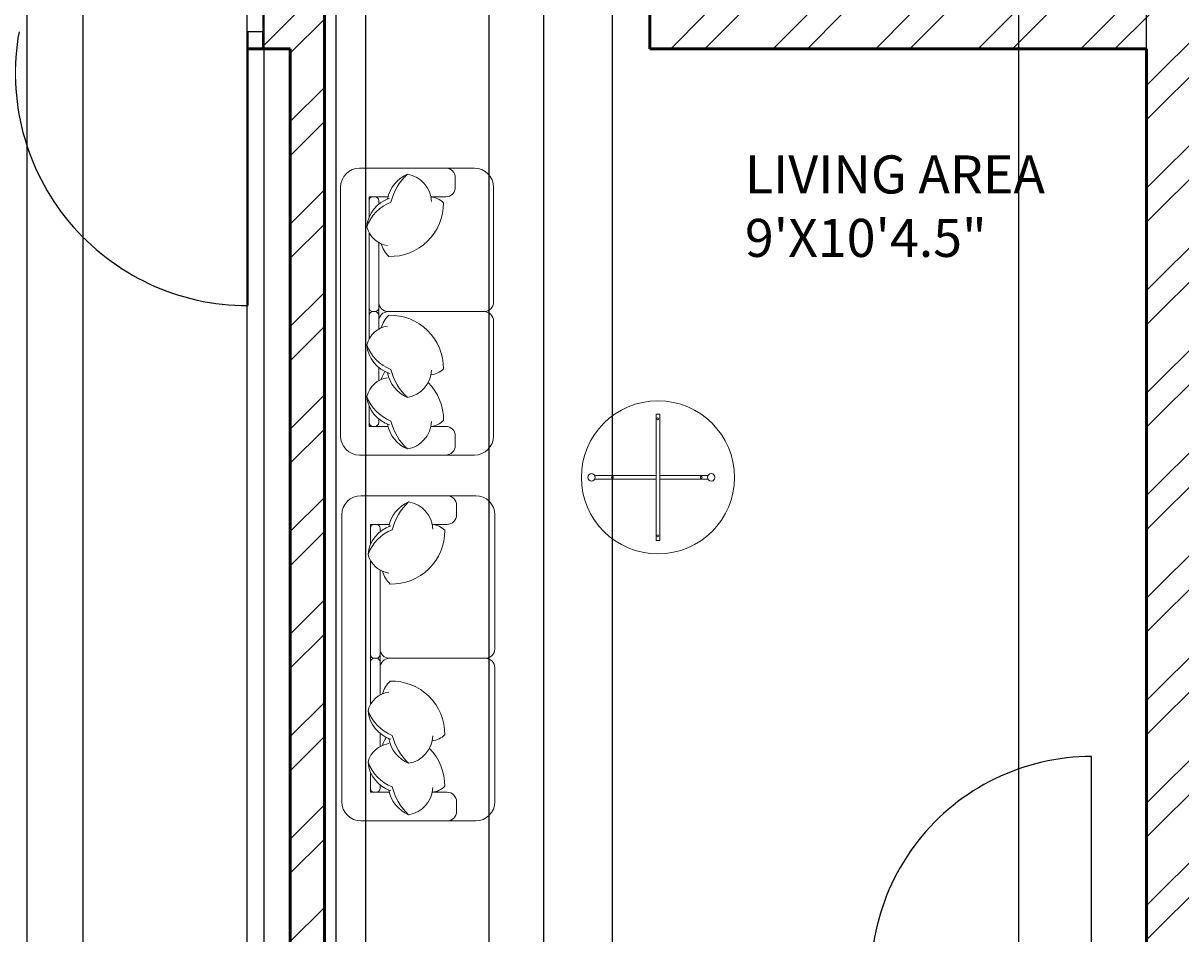
# Model space of a CAD drawing. Units: inches. Extents: x 1980 to 2738, y 1471 to 2568.
# Tile 17 of 22: x 2211 to 2363, y 2112 to 2232. Entities that reach past the tile are written whole.
import ezdxf

# ---------------------------------------------------------------- set-up
doc = ezdxf.new("R2010")
doc.units = ezdxf.units.IN
for name, color, linetype, lineweight in [('A-ANNO-DIMS', 2, 'Continuous', 18), ('A-AREA-IDEN', 7, 'Continuous', 18), ('A-DOOR', 31, 'Continuous', 25), ('A-FURN', 8, 'Continuous', 18), ('A-WALL', 7, 'Continuous', 50)]:
    doc.layers.add(name, color=color, linetype=linetype, lineweight=lineweight)
doc.layers.add('A-WALL-PATT', color=9, linetype='Continuous', lineweight=13, true_color=0xd19cc7)
doc.styles.get("Standard").update_dxf_attribs({"font": 'arial.ttf'})
doc.dimstyles.get("Standard").update_dxf_attribs({"dimtxt": 0.18, "dimasz": 0.18, "dimexe": 0.18, "dimexo": 0.0625, "dimgap": 0.09, "dimtad": 0, "dimtih": 1, "dimtoh": 1, "dimdec": 4, "dimzin": 0, "dimdsep": 46, "dimtxsty": 'Standard', "dimcen": 0.09, "dimadec": 0, "dimazin": 0, "dimtfac": 1, "dimtdec": 4, "dimtofl": 0, "dimtmove": 0, "dimatfit": 3, "dimfxl": 1, "dimtolj": 1, "dimtzin": 0, "dimarcsym": 0})

# ---------------------------------------------------------------- blocks, each defined once
blk = doc.blocks.new('table r 343')
at = {"color": 0}
for p, q in [((-10, 10), (-10, 262.1)), ((10, 10), (10, 262.1)), ((-330.3, 10), (330.3, 10)), ((-330.3, 10), (-330.3, -10)), ((330.3, 10), (330.3, -10)), ((-330.3, -10), (330.3, -10)), ((-10, -330.3), (-10, -10)), ((10, -330.3), (10, -10))]:
    blk.add_line(p, q, dxfattribs=at)
for centre, radius in [((0, 0), 400), ((0, 278.7), 19.4), ((0, 226.8), 5), ((-306.1, 0), 5), ((306.1, 0), 5), ((0, -238.1), 5), ((0, -346.9), 19.4)]:
    blk.add_circle(centre, radius, dxfattribs=at)
blk = doc.blocks.new('*D44')
at = {"layer": 'A-ANNO-DIMS', "color": 0, "lineweight": -2, "transparency": 16777216}
for p, q in [((2218.88, 1694.77), (2218.88, 2507.54)), ((2219.06, 2507.36), (2229.18, 2507.36)), ((2240.22, 2507.36), (2230.11, 2507.36)), ((2240.4, 1694.77), (2240.4, 2507.54))]:
    blk.add_line(p, q, dxfattribs=at)
at = {"layer": 'A-ANNO-DIMS', "color": 0, "transparency": 16777216}
for points in [[(2219.06, 2507.39), (2219.06, 2507.33), (2218.88, 2507.36)], [(2240.22, 2507.39), (2240.22, 2507.33), (2240.4, 2507.36)]]:
    blk.add_solid(points, dxfattribs=at)
at = {"layer": 'Defpoints', "color": 0, "transparency": 16777216}
for p in [(2240.4, 2507.36), (2218.88, 1694.71), (2240.4, 1694.71)]:
    blk.add_point(p, dxfattribs=at)
at = {"layer": 'A-ANNO-DIMS', "color": 0, "transparency": 16777216, "insert": (2229.64, 2507.36), "char_height": 0.18, "attachment_point": 5}
blk.add_mtext('\\A1;21.525', dxfattribs=at)
blk = doc.blocks.new('*D45')
at = {"layer": 'A-ANNO-DIMS', "color": 0, "lineweight": -2, "transparency": 16777216}
for p, q in [((2255.99, 1694.77), (2255.99, 2507.54)), ((2256.17, 2507.36), (2267.22, 2507.36)), ((2279.21, 2507.36), (2268.15, 2507.36)), ((2279.39, 1694.77), (2279.39, 2507.54))]:
    blk.add_line(p, q, dxfattribs=at)
at = {"layer": 'A-ANNO-DIMS', "color": 0, "transparency": 16777216}
for points in [[(2256.17, 2507.39), (2256.17, 2507.33), (2255.99, 2507.36)], [(2279.21, 2507.39), (2279.21, 2507.33), (2279.39, 2507.36)]]:
    blk.add_solid(points, dxfattribs=at)
at = {"layer": 'Defpoints', "color": 0, "transparency": 16777216}
for p in [(2279.39, 2507.36), (2255.99, 1694.71), (2279.39, 1694.71)]:
    blk.add_point(p, dxfattribs=at)
at = {"layer": 'A-ANNO-DIMS', "color": 0, "transparency": 16777216, "insert": (2267.69, 2507.36), "char_height": 0.18, "attachment_point": 5}
blk.add_mtext('\\A1;23.407', dxfattribs=at)
blk = doc.blocks.new('*D46')
at = {"layer": 'A-ANNO-DIMS', "color": 0, "lineweight": -2, "transparency": 16777216}
for p, q in [((2211.52, 1814.77), (2211.52, 2507.54)), ((2211.7, 2507.36), (2226.69, 2507.36)), ((2242.46, 2507.36), (2227.48, 2507.36)), ((2242.64, 1814.77), (2242.64, 2507.54))]:
    blk.add_line(p, q, dxfattribs=at)
at = {"layer": 'A-ANNO-DIMS', "color": 0, "transparency": 16777216}
for points in [[(2211.7, 2507.39), (2211.7, 2507.33), (2211.52, 2507.36)], [(2242.46, 2507.39), (2242.46, 2507.33), (2242.64, 2507.36)]]:
    blk.add_solid(points, dxfattribs=at)
at = {"layer": 'Defpoints', "color": 0, "transparency": 16777216}
for p in [(2242.64, 2507.36), (2211.52, 1814.71), (2242.64, 1814.71)]:
    blk.add_point(p, dxfattribs=at)
at = {"layer": 'A-ANNO-DIMS', "color": 0, "transparency": 16777216, "insert": (2227.08, 2507.36), "char_height": 0.18, "attachment_point": 5}
blk.add_mtext('\\A1;31.12', dxfattribs=at)
blk = doc.blocks.new('*D50')
at = {"layer": 'A-ANNO-DIMS', "color": 0, "lineweight": -2, "transparency": 16777216}
for p, q in [((2288.43, 1708.09), (2288.43, 2507.54)), ((2288.61, 2507.36), (2314.71, 2507.36)), ((2341.6, 2507.36), (2315.5, 2507.36)), ((2341.78, 1708.09), (2341.78, 2507.54))]:
    blk.add_line(p, q, dxfattribs=at)
at = {"layer": 'A-ANNO-DIMS', "color": 0, "transparency": 16777216}
for points in [[(2288.61, 2507.39), (2288.61, 2507.33), (2288.43, 2507.36)], [(2341.6, 2507.39), (2341.6, 2507.33), (2341.78, 2507.36)]]:
    blk.add_solid(points, dxfattribs=at)
at = {"layer": 'Defpoints', "color": 0, "transparency": 16777216}
for p in [(2341.78, 2507.36), (2288.43, 1708.03), (2341.78, 1708.03)]:
    blk.add_point(p, dxfattribs=at)
at = {"layer": 'A-ANNO-DIMS', "color": 0, "transparency": 16777216, "insert": (2315.11, 2507.36), "char_height": 0.18, "attachment_point": 5}
blk.add_mtext('\\A1;53.34', dxfattribs=at)
blk = doc.blocks.new('*D51')
at = {"layer": 'A-ANNO-DIMS', "color": 0, "lineweight": -2, "transparency": 16777216}
for p, q in [((2341.78, 1708.09), (2341.78, 2507.54)), ((2341.96, 2507.36), (2349.72, 2507.36)), ((2358.4, 2507.36), (2350.63, 2507.36)), ((2358.58, 1694.77), (2358.58, 2507.54))]:
    blk.add_line(p, q, dxfattribs=at)
at = {"layer": 'A-ANNO-DIMS', "color": 0, "transparency": 16777216}
for points in [[(2341.96, 2507.39), (2341.96, 2507.33), (2341.78, 2507.36)], [(2358.4, 2507.39), (2358.4, 2507.33), (2358.58, 2507.36)]]:
    blk.add_solid(points, dxfattribs=at)
at = {"layer": 'Defpoints', "color": 0, "transparency": 16777216}
for p in [(2358.58, 2507.36), (2341.78, 1708.03), (2358.58, 1694.71)]:
    blk.add_point(p, dxfattribs=at)
at = {"layer": 'A-ANNO-DIMS', "color": 0, "transparency": 16777216, "insert": (2350.18, 2507.36), "char_height": 0.18, "attachment_point": 5}
blk.add_mtext('\\A1;16.807', dxfattribs=at)
blk = doc.blocks.new('*D54')
at = {"layer": 'A-ANNO-DIMS', "color": 0, "lineweight": -2, "transparency": 16777216}
for p, q in [((2252.1, 1949.01), (2252.1, 2507.54)), ((2252.28, 2507.36), (2261.78, 2507.36)), ((2272.03, 2507.36), (2262.53, 2507.36)), ((2272.21, 1949.01), (2272.21, 2507.54))]:
    blk.add_line(p, q, dxfattribs=at)
at = {"layer": 'A-ANNO-DIMS', "color": 0, "transparency": 16777216}
for points in [[(2252.28, 2507.39), (2252.28, 2507.33), (2252.1, 2507.36)], [(2272.03, 2507.39), (2272.03, 2507.33), (2272.21, 2507.36)]]:
    blk.add_solid(points, dxfattribs=at)
at = {"layer": 'Defpoints', "color": 0, "transparency": 16777216}
for p in [(2272.21, 2507.36), (2252.1, 1948.95), (2272.21, 1948.95)]:
    blk.add_point(p, dxfattribs=at)
at = {"layer": 'A-ANNO-DIMS', "color": 0, "transparency": 16777216, "insert": (2262.16, 2507.36), "char_height": 0.18, "attachment_point": 5}
blk.add_mtext('\\A1;20.11', dxfattribs=at)

msp = doc.modelspace()

# ---------------------------------------------------------------- hatches: boundary and pattern name
at = {"layer": 'A-WALL-PATT'}
h = msp.add_hatch(dxfattribs=at)
h.set_pattern_fill('ANSI32', color=256)
h.paths.add_polyline_path([(2257.5661, 2416.2064), (2257.5661, 2420.7064), (2250.5833, 2420.7064), (2250.5833, 2462.7064), (2246.0833, 2462.7064), (2246.0833, 2420.7064), (2237.0791, 2420.7064), (2237.0791, 2411.7064), (2246.0833, 2411.7064), (2246.0833, 2291.7064), (2242.6109, 2291.7064), (2242.6109, 2287.2064), (2246.0833, 2287.2064), (2250.5833, 2287.2064), (2250.5833, 2291.7064), (2250.5833, 2411.7064), (2257.5661, 2411.7064)])
h.paths.add_polyline_path([(2387.0396, 2416.2064), (2387.0396, 2420.7064), (2367.5833, 2420.7064), (2367.5833, 2462.7064), (2358.5833, 2462.7064), (2358.5833, 2420.7064), (2329.3087, 2420.7064), (2329.3087, 2411.7064), (2358.5833, 2411.7064), (2358.5833, 2321.7275), (2358.5833, 2309.7064), (2347.3089, 2309.7064), (2293.3089, 2309.7064), (2293.3089, 2259.0771), (2297.8089, 2259.0771), (2297.8089, 2305.2064), (2347.3089, 2305.2064), (2347.3089, 2284.7412), (2351.8089, 2284.7412), (2351.8089, 2305.2064), (2372.3188, 2305.2064), (2372.3761, 2284.3899), (2377.0295, 2284.3899), (2377.0295, 2299.3058), (2377.0295, 2305.2064), (2426.5295, 2305.2064), (2426.5295, 2257.5573), (2431.0295, 2257.5573), (2431.0295, 2309.7064), (2377.0295, 2309.7064), (2367.5833, 2309.7064), (2367.5833, 2321.7275), (2367.5833, 2411.7064), (2387.0396, 2411.7064)])
h.paths.add_polyline_path([(2448.5267, 2416.2064), (2448.5267, 2420.7064), (2423.0396, 2420.7064), (2423.0396, 2411.7064), (2448.5267, 2411.7064)])
h.paths.add_polyline_path([(2130.9128, 2416.2064), (2130.9128, 2420.7064), (2105.0833, 2420.7064), (2105.0833, 2386.6942), (2114.0833, 2386.6942), (2114.0833, 2411.7064), (2130.9128, 2411.7064)])
h.paths.add_polyline_path([(2212.9478, 2420.7064), (2190.9128, 2420.7064), (2190.9128, 2411.7064), (2212.9478, 2411.7064), (2212.9478, 2416.2064)])
h.paths.add_polyline_path([(2114.0833, 2326.6942), (2105.0833, 2326.6942), (2105.0833, 2291.7064), (2081.0833, 2291.7064), (2081.0833, 2287.2064), (2105.0833, 2287.2064), (2105.0833, 2276.1935), (2114.0833, 2276.1935), (2114.0833, 2287.2064), (2166.3825, 2287.2064), (2166.3825, 2289.4564), (2166.3825, 2291.7064), (2114.0833, 2291.7064)])
h.paths.add_polyline_path([(2114.0833, 2252.1935), (2105.0833, 2252.1935), (2105.0833, 2233.2064), (2081.0833, 2233.2064), (2081.0833, 2228.7064), (2105.0833, 2228.7064), (2105.0833, 2213.4478), (2114.0833, 2213.4478), (2114.0833, 2228.7064), (2195.0833, 2228.7064), (2199.5833, 2228.7064), (2208.4455, 2228.7064), (2208.4455, 2230.9564), (2208.4455, 2233.2064), (2199.5833, 2233.2064), (2199.5833, 2287.2064), (2206.8904, 2287.2064), (2206.8904, 2289.4564), (2206.8904, 2291.7064), (2189.446, 2291.7064), (2189.446, 2289.4564), (2189.446, 2287.2064), (2195.0833, 2287.2064), (2195.0833, 2233.2064), (2114.0833, 2233.2064)])
h.paths.add_polyline_path([(2114.0833, 2153.4478), (2109.5833, 2153.4478), (2105.0833, 2153.4478), (2105.0833, 2135.2374), (2114.0833, 2135.2374)], flags=17)
h.paths.add_polyline_path([(2135.9619, 2095.4081), (2140.1805, 2095.4081), (2140.1805, 2104.2064), (2114.0833, 2104.2064), (2114.0833, 2110.3997), (2109.5833, 2110.3997), (2105.0833, 2110.3997), (2105.0833, 2104.2064), (2081.0833, 2104.2064), (2081.0833, 2099.7064), (2105.0833, 2099.7064), (2127.5416, 2099.8532), (2127.5416, 2056.9393), (2136.2133, 2056.9393)], flags=17)
h.paths.add_polyline_path([(2255.4895, 2104.2064), (2250.5833, 2104.2064), (2250.5833, 2233.2064), (2246.0833, 2233.2064), (2242.4941, 2233.2064), (2242.4941, 2228.7064), (2246.0833, 2228.7064), (2246.0833, 2104.2064), (2163.6825, 2104.2064), (2163.6825, 2099.8072), (2163.6825, 2095.4081), (2191.4325, 2095.4081), (2191.4325, 2011.2064), (2186.0833, 2011.2064), (2136.5143, 2010.8824), (2136.3702, 2032.9403), (2131.9559, 2032.9115), (2127.5416, 2032.8826), (2127.5416, 2006.7064), (2105.0833, 2006.7064), (2081.0833, 2006.7064), (2081.0833, 2002.2064), (2105.0833, 2002.2064), (2105.0833, 1995.9329), (2114.0833, 1995.9329), (2114.0833, 2002.2064), (2246.0833, 2002.2064), (2246.0833, 1877.7064), (2242.1358, 1877.7064), (2242.1358, 1873.2064), (2250.5833, 1873.2064), (2250.5833, 2002.2064), (2255.3335, 2002.2064), (2255.3335, 2011.2064), (2195.9325, 2011.2064), (2195.9325, 2095.2064), (2255.4895, 2095.2064), (2255.4895, 2099.5471)])
h.paths.add_polyline_path([(2199.5833, 1873.2064), (2209.827, 1873.2064), (2209.827, 1875.4564), (2209.827, 1877.7064), (2114.0833, 1877.7064), (2114.0833, 1890.0968), (2105.0833, 1890.0968), (2105.0833, 1877.7064), (2081.0833, 1877.7064), (2081.0833, 1873.2064), (2105.0833, 1873.2064), (2105.0833, 1857.7279), (2114.0833, 1857.7279), (2114.0833, 1873.2064), (2195.0833, 1873.2064), (2195.0833, 1819.2064), (2190.298, 1819.2064), (2190.298, 1814.7064), (2209.8976, 1814.7064), (2209.8976, 1816.9564), (2209.8976, 1819.2064), (2199.5833, 1819.2064)])
h.paths.add_polyline_path([(2114.0833, 1814.7064), (2166.2538, 1814.7064), (2166.2538, 1816.9564), (2166.2538, 1819.2064), (2114.0833, 1819.2064), (2114.0833, 1833.7279), (2109.5833, 1833.7279), (2105.0833, 1833.7279), (2105.0833, 1819.2064), (2081.0833, 1819.2064), (2081.0833, 1814.7064), (2105.0833, 1814.7064), (2105.0833, 1782.5516), (2114.0833, 1782.5516)])
h.paths.add_polyline_path([(2114.0833, 1722.5516), (2109.5833, 1722.5516), (2105.0833, 1722.5516), (2105.0833, 1685.7064), (2124.5104, 1685.7064), (2124.5104, 1690.2064), (2124.5104, 1694.7064), (2114.0833, 1694.7064)])
h.paths.add_polyline_path([(2218.8787, 1694.7064), (2184.5104, 1694.7064), (2184.5104, 1685.7064), (2218.8787, 1685.7064), (2218.8787, 1690.2064)])
h.paths.add_polyline_path([(2250.5833, 1819.2064), (2242.6431, 1819.2064), (2242.6431, 1816.9564), (2242.6431, 1814.7064), (2246.0833, 1814.7064), (2246.0833, 1694.7064), (2240.4035, 1694.7064), (2240.4035, 1690.2064), (2240.4035, 1685.7064), (2246.0833, 1685.7064), (2246.0833, 1643.7064), (2250.5833, 1643.7064), (2250.5833, 1685.7064), (2255.9859, 1685.7064), (2255.9859, 1690.2064), (2255.9859, 1694.7064), (2250.5833, 1694.7064)])
h.paths.add_polyline_path([(2297.4764, 1694.7064), (2279.3934, 1694.7064), (2279.3934, 1690.2064), (2279.3934, 1685.7064), (2297.4764, 1685.7064), (2297.4764, 1690.2064)])
h.paths.add_polyline_path([(2377.1596, 1694.7064), (2367.5833, 1694.7064), (2367.5833, 1787.7064), (2431.0295, 1787.7064), (2431.0295, 1792.2064), (2431.0295, 1849.4149), (2428.7795, 1849.4149), (2426.5295, 1849.4149), (2426.5295, 1792.2064), (2421.5833, 1792.2064), (2367.5833, 1792.2064), (2297.8089, 1792.2064), (2297.8089, 1850.2946), (2295.5589, 1850.2946), (2293.3089, 1850.2946), (2293.3089, 1792.2064), (2293.3089, 1787.7064), (2297.8089, 1787.7064), (2358.5833, 1787.7064), (2358.5833, 1694.7064), (2333.4764, 1694.7064), (2333.4764, 1685.7064), (2358.5833, 1685.7064), (2358.5833, 1643.7064), (2367.5833, 1643.7064), (2367.5833, 1685.7064), (2377.1596, 1685.7064)])
h.paths.add_polyline_path([(2442.4912, 1694.7064), (2413.1596, 1694.7064), (2413.1596, 1685.7064), (2442.4912, 1685.7064)])
h.paths.add_polyline_path([(2480.0833, 1814.7064), (2483.4816, 1814.7064), (2483.4816, 1817.9384), (2483.4816, 1819.2064), (2475.5833, 1819.2064), (2475.5833, 1694.7064), (2470.7283, 1694.7064), (2470.7283, 1685.7064), (2475.5833, 1685.7064), (2475.5833, 1643.7064), (2480.0833, 1643.7064), (2480.0833, 1685.7064), (2486.3293, 1685.7064), (2486.3293, 1690.2064), (2486.3293, 1694.7064), (2480.0833, 1694.7064)])
h.paths.add_polyline_path([(2621.0833, 1721.7349), (2612.0833, 1721.7349), (2612.0833, 1694.7064), (2586.1453, 1694.7064), (2586.1453, 1685.7064), (2621.0833, 1685.7064)])
h.paths.add_polyline_path([(2526.1453, 1690.2064), (2526.1453, 1694.7064), (2511.584, 1694.7064), (2511.584, 1690.2064), (2511.584, 1685.7064), (2526.1453, 1685.7064)])
h.paths.add_polyline_path([(2645.0833, 1819.2064), (2621.0833, 1819.2064), (2621.0833, 1835.8527), (2616.5833, 1835.8527), (2612.0833, 1835.8527), (2612.0833, 1819.2064), (2560.2541, 1819.2064), (2560.2541, 1814.7064), (2612.0833, 1814.7064), (2612.0833, 1781.7349), (2621.0833, 1781.7349), (2621.0833, 1814.7064), (2645.0833, 1814.7064)])
h.paths.add_polyline_path([(2645.0833, 1877.7064), (2621.0833, 1877.7064), (2621.0833, 1886.4375), (2612.0833, 1886.4375), (2612.0833, 1877.7064), (2517.1032, 1877.7064), (2517.1032, 1875.4564), (2517.1032, 1873.2064), (2526.5833, 1873.2064), (2526.5833, 1819.2064), (2516.6454, 1819.2064), (2516.6454, 1816.9564), (2516.6454, 1814.7064), (2536.4445, 1814.7064), (2536.4445, 1816.9564), (2536.4445, 1819.2064), (2531.0833, 1819.2064), (2531.0833, 1873.2064), (2612.0833, 1873.2064), (2612.0833, 1859.8527), (2621.0833, 1859.8527), (2621.0833, 1873.2064), (2645.0833, 1873.2064)])
h.paths.add_polyline_path([(2645.0833, 2006.7064), (2621.0833, 2006.7064), (2588.5085, 2006.7064), (2588.5085, 2052.9125), (2579.9045, 2052.9125), (2579.9045, 2011.2064), (2519.9045, 2011.2064), (2519.9045, 2095.2064), (2553.1204, 2095.2064), (2553.1204, 2104.2064), (2480.0833, 2104.2064), (2480.0833, 2228.7064), (2484.3832, 2228.7064), (2484.3832, 2230.9564), (2484.3832, 2233.2064), (2475.5833, 2233.2064), (2475.5833, 2104.2064), (2463.1308, 2104.2064), (2463.1308, 2095.2064), (2501.2463, 2095.2064), (2510.9045, 2095.2064), (2515.4045, 2095.2064), (2515.4045, 2011.2064), (2510.9045, 2011.2064), (2501.2463, 2011.2064), (2462.5957, 2011.2064), (2462.5957, 2002.2064), (2475.5833, 2002.2064), (2475.5833, 1873.2064), (2483.6146, 1873.2064), (2483.6146, 1875.4564), (2483.6146, 1877.7064), (2480.0833, 1877.7064), (2480.0833, 2002.2064), (2612.0833, 2002.2064), (2612.0833, 1996.309), (2621.0833, 1996.309), (2621.0833, 2002.2064), (2645.0833, 2002.2064)])
h.paths.add_polyline_path([(2588.5085, 2099.7277), (2621.0833, 2099.7277), (2645.0833, 2099.7064), (2645.0833, 2104.2064), (2621.0833, 2104.2064), (2621.0833, 2109.0038), (2616.5833, 2109.0038), (2612.0833, 2109.0038), (2612.0833, 2104.2064), (2575.0621, 2104.2064), (2575.0621, 2099.7064), (2575.0621, 2095.2064), (2579.9045, 2095.2064), (2579.9045, 2076.9125), (2588.5085, 2076.9125)], flags=17)
h.paths.add_polyline_path([(2367.5833, 2002.2064), (2373.7228, 2002.2064), (2373.7228, 2006.7064), (2373.7228, 2011.2064), (2350.7889, 2011.2064), (2350.7889, 2006.7064), (2350.7889, 2002.2064), (2358.5833, 2002.2064), (2358.5833, 1877.7064), (2293.3089, 1877.7064), (2293.3089, 1870.4987), (2297.8089, 1870.4987), (2297.8089, 1873.2064), (2347.3089, 1873.2064), (2347.3089, 1847.2208), (2351.8089, 1847.2208), (2351.8089, 1873.2064), (2372.5295, 1873.2064), (2372.5295, 1847.8619), (2377.0295, 1847.8619), (2377.0295, 1873.2064), (2426.5295, 1873.2064), (2426.5295, 1868.7339), (2431.0295, 1868.7339), (2431.0295, 1877.7064), (2367.5833, 1877.7064)])
h.paths.add_polyline_path([(2531.0833, 2287.2064), (2534.2285, 2287.2064), (2534.2285, 2291.7064), (2516.7886, 2291.7064), (2516.7886, 2287.2064), (2526.5833, 2287.2064), (2526.5833, 2233.2064), (2517.9112, 2233.2064), (2517.9112, 2230.9564), (2517.9112, 2228.7064), (2526.5833, 2228.7064), (2531.0833, 2228.7064), (2612.0833, 2228.7064), (2612.0833, 2206.8504), (2621.0833, 2206.8504), (2621.0833, 2228.7064), (2645.0833, 2228.7064), (2645.0833, 2233.2064), (2621.0833, 2233.2064), (2621.0833, 2241.8536), (2616.5833, 2241.8536), (2612.0833, 2241.8536), (2612.0833, 2233.2064), (2531.0833, 2233.2064)])
h.paths.add_polyline_path([(2645.0833, 2291.7064), (2621.0833, 2291.7064), (2621.0833, 2323.0138), (2616.5833, 2323.0138), (2612.0833, 2323.0138), (2612.0833, 2291.7064), (2559.6852, 2291.7064), (2559.6852, 2289.4564), (2559.6852, 2287.2064), (2612.0833, 2287.2064), (2612.0833, 2265.8536), (2621.0833, 2265.8536), (2621.0833, 2287.2064), (2645.0833, 2287.2064)])
h.paths.add_polyline_path([(2621.0833, 2420.7064), (2582.8189, 2420.7064), (2582.8189, 2411.7064), (2612.0833, 2411.7064), (2612.0833, 2383.0138), (2621.0833, 2383.0138)])
h.paths.add_polyline_path([(2480.0833, 2411.7064), (2485.7342, 2411.7064), (2485.7342, 2416.2064), (2485.7342, 2420.7064), (2480.0833, 2420.7064), (2480.0833, 2462.7064), (2475.5833, 2462.7064), (2475.5833, 2420.7064), (2469.4083, 2420.7064), (2469.4083, 2411.7064), (2475.5833, 2411.7064), (2475.5833, 2291.7064), (2475.5833, 2287.2064), (2482.9195, 2287.2064), (2482.9195, 2289.4564), (2482.9195, 2291.7064), (2480.0833, 2291.7064)])
h.paths.add_polyline_path([(2367.5833, 2228.7064), (2431.0295, 2228.7064), (2431.0295, 2233.2064), (2431.0295, 2237.4203), (2428.7795, 2237.4203), (2426.5295, 2237.4203), (2426.5295, 2233.2064), (2377.0295, 2233.2064), (2377.0295, 2260.3837), (2372.4423, 2260.3837), (2372.517, 2233.2635), (2351.8089, 2233.2064), (2351.8089, 2260.7412), (2347.3089, 2260.7412), (2347.3089, 2233.2064), (2297.8089, 2233.2064), (2297.8089, 2236.9324), (2293.3089, 2236.9324), (2293.3089, 2228.7064), (2358.5833, 2228.7064), (2358.5833, 2104.2064), (2353.3665, 2104.2064), (2353.3665, 2095.2064), (2373.8869, 2095.2064), (2373.8869, 2099.7064), (2373.8869, 2104.2064), (2367.5833, 2104.2064)])
h.paths.add_polyline_path([(2321.2323, 2104.2064), (2303.4895, 2104.2064), (2303.4895, 2095.2064), (2321.2323, 2095.2064), (2321.2323, 2099.7064)], flags=0)
h.paths.add_polyline_path([(2415.1308, 2099.7064), (2415.1308, 2104.2064), (2404.81, 2104.2064), (2404.81, 2095.2064), (2415.1308, 2095.2064)], flags=17)
h.paths.add_polyline_path([(2318.6336, 2011.2064), (2303.3335, 2011.2064), (2303.3335, 2002.2064), (2318.6336, 2002.2064)], flags=0)
h.paths.add_polyline_path([(2414.5957, 2011.2064), (2406.2461, 2011.2064), (2406.2461, 2006.7064), (2406.2461, 2002.2064), (2414.5957, 2002.2064)], flags=17)

# ---------------------------------------------------------------- linework, layer by layer
at = {"layer": 'A-DOOR'}
for p, q in [((2242.4941, 2233.2064), (2242.4941, 2228.7064)), ((2242.4941, 2230.9564), (2240.4941, 2230.9564)), ((2240.4941, 2230.9564), (2240.4941, 2194.9564)), ((2242.4941, 2228.7064), (2242.4941, 2230.9564)), ((2351.3665, 2123.7064), (2351.3665, 2135.7064)), ((2351.3665, 2099.7064), (2351.3665, 2123.7064))]:
    msp.add_line(p, q, dxfattribs=at)
for centre, radius, start, end in [((2240.4941, 2225.4969), 30.5405, 169.702376, 270), ((2351.3665, 2106.7129), 28.9935, 90, 193.984358)]:
    msp.add_arc(centre, radius, start, end, dxfattribs=at)
at = {"layer": 'A-FURN', "ltscale": 0.03}
for points in [[(2272.7882, 2195.4307, -0.41421356), (2271.5313, 2194.1738, -0.41421356), (2272.7882, 2192.9169), (2272.7882, 2177.8339, -0.41421356), (2270.2744, 2175.32), (2255.1914, 2175.32, -0.41421356), (2252.6775, 2177.8339), (2252.6775, 2210.5137, -0.41421356), (2255.1914, 2213.0275), (2270.2744, 2213.0275, -0.41421356), (2272.7882, 2210.5137), (2272.7882, 2195.4307, -0.41421356), (2271.5313, 2194.1738, -0.41421356), (2272.7882, 2192.9169)], [(2272.9571, 2149.8668, -0.41421356), (2271.7001, 2148.6099, -0.41421356), (2272.9571, 2147.353), (2272.9571, 2129.7561, -0.41421356), (2270.4432, 2127.2423), (2255.3602, 2127.2423, -0.41421356), (2252.8464, 2129.7561), (2252.8464, 2167.4636, -0.41421356), (2255.3602, 2169.9775), (2270.4432, 2169.9775, -0.41421356), (2272.9571, 2167.4636), (2272.9571, 2149.8668, -0.41421356), (2271.7001, 2148.6099, -0.41421356), (2272.9571, 2147.353)]]:
    msp.add_lwpolyline(points, format="xyb", dxfattribs=at)
at = {"layer": 'A-FURN'}
for points in [[(2261.4641, 2212.2276, 0.14772988), (2259.3039, 2208.554, 0.21334276), (2256.1357, 2205.3126, 0.17866181)], [(2264.6323, 2208.626, 0.35677236), (2261.4641, 2212.2276, 0.24954205), (2258.8532, 2208.9642, -9.61688035)], [(2266.5036, 2213.0275, -0.41421356), (2267.7605, 2211.7706), (2267.7605, 2210.5137, -0.41421356), (2266.5036, 2209.2568), (2264.5562, 2209.2568)], [(2259.1318, 2209.0615, 0.30666349), (2256.1357, 2205.3126, 0.30632997), (2258.8719, 2202.8635, -0.87284716)], [(2257.7052, 2208.2976), (2257.7052, 2208.754, 0.41421356), (2257.2024, 2209.2568), (2256.951, 2209.2568, 0.41421356), (2256.4483, 2208.754)], [(2264.5556, 2209.2595, -0.16554063), (2266.2164, 2208.4819, -0.42598917), (2259.0159, 2201.4229, -0.12152332), (2258.0234, 2203.0985, 7.11546429)], [(2256.4483, 2204.5215), (2256.4483, 2194.6765, 0.41421356), (2256.951, 2194.1738), (2257.2024, 2194.1738, 0.41421356), (2257.7052, 2194.6765), (2257.7052, 2203.2559, 0.41421356)], [(2257.7052, 2195.4307, 0.41421356), (2258.9621, 2194.1738)], [(2257.7052, 2195.4307, 0.41421356), (2258.9621, 2194.1738), (2271.5313, 2194.1738, 0.41421356)], [(2256.4483, 2190.597), (2256.4483, 2193.671, -0.41421356), (2256.951, 2194.1738), (2257.2024, 2194.1738, -0.41421356), (2257.7052, 2193.671), (2257.7052, 2191.8626, -0.41421356)], [(2257.7052, 2192.9169, -0.41421356), (2258.9621, 2194.1738)], [(2257.7052, 2192.9169, -0.41421356), (2258.9621, 2194.1738), (2271.5313, 2194.1738, -0.41421356)], [(2264.5556, 2185.859, 0.16554063), (2266.2164, 2186.6366, 0.42598917), (2259.0159, 2193.6957, 0.12152332), (2258.0234, 2192.02, -7.11546429)], [(2259.1318, 2186.057, -0.30666349), (2256.1357, 2189.806, -0.30632997), (2258.8719, 2192.255, 0.87284716)], [(2261.4641, 2182.8909, -0.14772988), (2259.3039, 2186.5645, -0.21334276), (2256.1357, 2189.806, -0.17866181)], [(2257.7052, 2186.8209), (2257.7052, 2185.0917, -0.41421356)], [(2258.5148, 2186.3028, 0.07186538), (2258.0234, 2185.249, -7.11546429)], [(2264.6323, 2186.4925, -0.35677236), (2261.4641, 2182.8909, -0.24954205), (2258.8532, 2186.1543, 9.61688035)], [(2259.1318, 2179.2861, -0.30666349), (2256.1357, 2183.035, -0.30632997), (2258.8719, 2185.4841, 0.87284716)], [(2264.5556, 2179.088, 0.16554063), (2266.2164, 2179.8656, 0.20023115), (2264.1937, 2184.8551, 0.12152332)], [(2261.4641, 2176.12, -0.14772988), (2259.3039, 2179.7936, -0.21334276), (2256.1357, 2183.035, -0.17866181)], [(2256.4483, 2181.735), (2256.4483, 2179.0908), (2258.9184, 2179.0908, -0.41421356)], [(2257.7052, 2180.0499), (2257.7052, 2179.5935, -0.41421356), (2257.2024, 2179.0908), (2256.951, 2179.0908, -0.41421356), (2256.4483, 2179.5935)], [(2264.6323, 2179.7215, -0.35677236), (2261.4641, 2176.12, -0.24954205), (2258.8532, 2179.3833, 9.61688035)], [(2264.5562, 2179.0908), (2266.5036, 2179.0908, -0.41421356), (2267.7605, 2177.8339), (2267.7605, 2176.5769, -0.41421356), (2266.5036, 2175.32)], [(2261.6329, 2169.1775, 0.14772988), (2259.4728, 2165.5039, 0.21334276), (2256.3046, 2162.2625, 0.17866181)], [(2264.8011, 2165.576, 0.35677236), (2261.6329, 2169.1775, 0.24954205), (2259.022, 2165.9142, -9.61688035)], [(2266.6725, 2169.9775, -0.41421356), (2267.9294, 2168.7206), (2267.9294, 2167.4636, -0.41421356), (2266.6725, 2166.2067), (2264.7251, 2166.2067)], [(2259.3006, 2166.0114, 0.30666349), (2256.3046, 2162.2625, 0.30632997), (2259.0407, 2159.8134, -0.87284716)], [(2257.8741, 2165.2475), (2257.8741, 2165.704, 0.41421356), (2257.3713, 2166.2067), (2257.1199, 2166.2067, 0.41421356), (2256.6171, 2165.704)], [(2264.7245, 2166.2095, -0.16554063), (2266.3852, 2165.4319, -0.42598917), (2259.1848, 2158.3728, -0.12152332), (2258.1923, 2160.0485, 7.11546429)], [(2256.6171, 2161.4715), (2256.6171, 2149.1126, 0.41421356), (2257.1199, 2148.6099), (2257.3713, 2148.6099, 0.41421356), (2257.8741, 2149.1126), (2257.8741, 2160.2058, 0.41421356)], [(2257.8741, 2149.8668, 0.41421356), (2259.131, 2148.6099)], [(2257.8741, 2149.8668, 0.41421356), (2259.131, 2148.6099), (2271.7001, 2148.6099, 0.41421356)], [(2256.6171, 2142.5193), (2256.6171, 2148.1071, -0.41421356), (2257.1199, 2148.6099), (2257.3713, 2148.6099, -0.41421356), (2257.8741, 2148.1071), (2257.8741, 2143.7849, -0.41421356)], [(2257.8741, 2147.353, -0.41421356), (2259.131, 2148.6099)], [(2257.8741, 2147.353, -0.41421356), (2259.131, 2148.6099), (2271.7001, 2148.6099, -0.41421356)], [(2264.7245, 2137.7813, 0.16554063), (2266.3852, 2138.5588, 0.42598917), (2259.1848, 2145.6179, 0.12152332), (2258.1923, 2143.9422, -7.11546429)], [(2259.3006, 2137.9793, -0.30666349), (2256.3046, 2141.7282, -0.30632997), (2259.0407, 2144.1773, 0.87284716)], [(2261.6329, 2134.8132, -0.14772988), (2259.4728, 2138.4868, -0.21334276), (2256.3046, 2141.7282, -0.17866181)], [(2257.8741, 2138.7432), (2257.8741, 2137.0139, -0.41421356)], [(2259.3006, 2131.2083, -0.30666349), (2256.3046, 2134.9573, -0.30632997), (2259.0407, 2137.4063, 0.87284716)], [(2258.6837, 2138.2251, 0.07186538), (2258.1923, 2137.1713, -7.11546429)], [(2264.8011, 2138.4148, -0.35677236), (2261.6329, 2134.8132, -0.24954205), (2259.022, 2138.0766, 9.61688035)], [(2264.7245, 2131.0103, 0.16554063), (2266.3852, 2131.7879, 0.20023115), (2264.3626, 2136.7774, 0.12152332)], [(2261.6329, 2128.0422, -0.14772988), (2259.4728, 2131.7158, -0.21334276), (2256.3046, 2134.9573, -0.17866181)], [(2256.6171, 2133.6572), (2256.6171, 2131.013), (2259.0873, 2131.013, -0.41421356)], [(2257.8741, 2131.9722), (2257.8741, 2131.5158, -0.41421356), (2257.3713, 2131.013), (2257.1199, 2131.013, -0.41421356), (2256.6171, 2131.5158)], [(2264.8011, 2131.6438, -0.35677236), (2261.6329, 2128.0422, -0.24954205), (2259.022, 2131.3056, 9.61688035)], [(2264.7251, 2131.013), (2266.6725, 2131.013, -0.41421356), (2267.9294, 2129.7561), (2267.9294, 2128.4992, -0.41421356), (2266.6725, 2127.2423)]]:
    msp.add_lwpolyline(points, format="xyb", dxfattribs=at)
for points in [[(2258.9184, 2209.2568), (2256.4483, 2209.2568), (2256.4483, 2206.6126)], [(2259.0873, 2166.2067), (2256.6171, 2166.2067), (2256.6171, 2163.5625)]]:
    msp.add_lwpolyline(points, dxfattribs=at)
for points in [[(2256.4483, 2194.6765), (2256.4483, 2193.671, -0.41421356), (2256.951, 2194.1738), (2257.2024, 2194.1738, -0.41421356), (2257.7052, 2193.671), (2257.7052, 2194.6765, -0.41421356), (2257.2024, 2194.1738), (2256.951, 2194.1738, -0.41421356)], [(2256.6171, 2149.1126), (2256.6171, 2148.1071, -0.41421356), (2257.1199, 2148.6099), (2257.3713, 2148.6099, -0.41421356), (2257.8741, 2148.1071), (2257.8741, 2149.1126, -0.41421356), (2257.3713, 2148.6099), (2257.1199, 2148.6099, -0.41421356)]]:
    msp.add_lwpolyline(points, format="xyb", close=True, dxfattribs=at)
at = {"layer": 'A-WALL'}
for p, q in [((2293.3089, 2236.9324), (2293.3089, 2228.7064)), ((2250.5833, 2233.2064), (2250.5833, 2104.2064)), ((2293.3089, 2228.7064), (2293.3089, 2233.2064)), ((2240.4941, 2228.7064), (2246.0833, 2228.7064)), ((2246.0833, 2228.7064), (2246.0833, 2104.2064)), ((2293.3089, 2228.7064), (2297.8089, 2228.7064)), ((2358.5833, 2228.7064), (2293.3089, 2228.7064)), ((2304.5833, 2228.7064), (2309.0833, 2228.7064)), ((2358.5833, 2228.7064), (2358.5833, 2104.2064))]:
    msp.add_line(p, q, dxfattribs=at)

# ---------------------------------------------------------------- block references
at = {"layer": 'A-FURN', "xscale": 0.0251383443972704, "yscale": 0.0251383443972704, "zscale": 0.0251383443972704, "rotation": 270}
msp.add_blockref('table r 343', (2294.38, 2172.3929), dxfattribs=at)

# ---------------------------------------------------------------- texts
at = {"layer": 'A-AREA-IDEN', "insert": (2305.8091, 2214.697), "char_height": 5, "attachment_point": 1}
msp.add_mtext_dynamic_manual_height_columns('LIVING AREA\\P9\'X10\'4.5"', width=136.915741, gutter_width=12.5, heights=[0], dxfattribs=at)

# ---------------------------------------------------------------- dimensions: what is measured, and where the dimension line sits
at = {"layer": 'A-ANNO-DIMS'}
for base, p1, p2, override, picture, middle in [((2242.6431, 2507.3564), (2211.5238, 1814.7064), (2242.6431, 1814.7064), {"dimdec": 2, "dimlfac": 1, "dimrnd": 0, "dimzin": 0, "dimdsep": 46, "dimlunit": 2}, '*D46', (2227.0835, 2507.3564)), ((2240.4035, 2507.3564), (2218.8787, 1694.7064), (2240.4035, 1694.7064), {"dimdec": 3, "dimlfac": 1, "dimrnd": 0, "dimzin": 0, "dimdsep": 46, "dimlunit": 2}, '*D44', (2229.6411, 2507.3564)), ((2272.2106, 2507.3564), (2252.1, 1948.9472), (2272.2106, 1948.9472), {"dimdec": 2, "dimlfac": 1, "dimrnd": 0, "dimzin": 0, "dimdsep": 46, "dimlunit": 2}, '*D54', (2262.1553, 2507.3564)), ((2279.39337, 2507.35642), (2255.98588, 1694.70642), (2279.39337, 1694.70642), {"dimdec": 3, "dimlfac": 1, "dimrnd": 0, "dimzin": 0, "dimdsep": 46, "dimlunit": 2}, '*D45', (2267.68962, 2507.35642)), ((2341.776, 2507.3564), (2288.4349, 1708.0291), (2341.776, 1708.0291), {"dimdec": 2, "dimlfac": 1, "dimrnd": 0, "dimzin": 0, "dimdsep": 46, "dimlunit": 2}, '*D50', (2315.1054, 2507.3564)), ((2358.5833, 2507.3564), (2341.776, 1708.0291), (2358.5833, 1694.7064), {"dimdec": 3, "dimlfac": 1, "dimrnd": 0, "dimzin": 0, "dimdsep": 46, "dimlunit": 2}, '*D51', (2350.1796, 2507.3564))]:
    dim = msp.add_linear_dim(base=base, p1=p1, p2=p2, dimstyle='Standard', override=override, dxfattribs=at)
    dim.commit()
    dim.dimension.update_dxf_attribs({"geometry": picture, "text_midpoint": middle})

doc.saveas('drawing.dxf')
